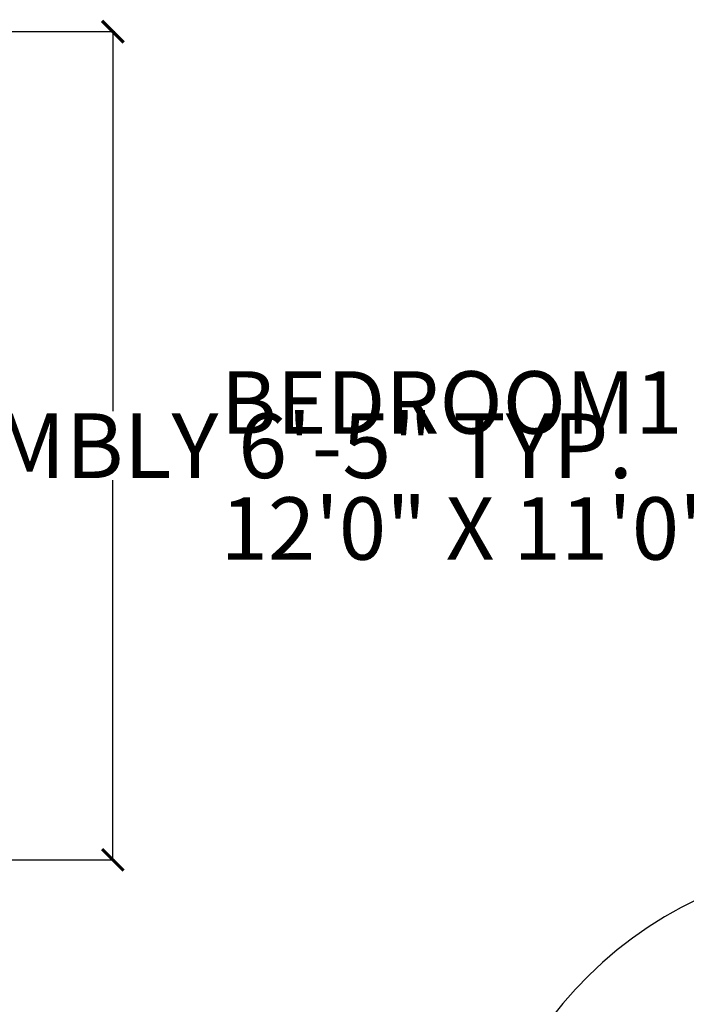
# Model space of a CAD drawing. Units: inches. Extents: x 528 to 2520, y -151 to 1354.
# Tile 6 of 41: x 658 to 720, y 1137 to 1229. Entities that reach past the tile are written whole.
import ezdxf

# ---------------------------------------------------------------- set-up
doc = ezdxf.new("R2010")
doc.units = ezdxf.units.IN
doc.header["$MEASUREMENT"] = 0
for name, color, linetype, lineweight in [('A-ANNO-DIMS', 2, 'Continuous', 18), ('A-AREA-IDEN', 7, 'Continuous', 18), ('A-Door', 150, 'Continuous', 25)]:
    doc.layers.add(name, color=color, linetype=linetype, lineweight=lineweight)
doc.layers.add('NT', color=1, linetype='Continuous')
doc.styles.get("Standard").update_dxf_attribs({"font": 'arial.ttf'})
doc.dimstyles.get("Standard").update_dxf_attribs({"dimtxt": 6, "dimasz": 2, "dimexe": 0.18, "dimexo": 0.0625, "dimgap": 0.09, "dimtad": 0, "dimtih": 1, "dimtoh": 1, "dimdec": 1, "dimzin": 0, "dimdsep": 46, "dimlunit": 3, "dimtxsty": 'Standard', "dimblk": 'ARCHTICK', "dimcen": 0.09, "dimadec": 0, "dimazin": 0, "dimtfac": 1, "dimtdec": 1, "dimtofl": 0, "dimtmove": 0, "dimatfit": 3, "dimfxl": 1, "dimtolj": 1, "dimtzin": 0, "dimarcsym": 0})

# ---------------------------------------------------------------- blocks, each defined once
blk = doc.blocks.new('A$C7DB75F4D')
at = {"layer": 'A-Door'}
for points in [[(625, 740), (625, 660), (665, 660), (665, 740)], [(625, 180), (625, 660), (665, 660), (665, 180)], [(625, 100), (625, 180), (665, 180), (665, 100)], [(35, 100), (35, 60), (50, 60), (50, 50), (50, 0), (0, 0), (0, 100)], [(665, 100), (700, 100), (700, 0), (650, 0), (650, 50), (650, 60), (665, 60)]]:
    blk.add_lwpolyline(points, close=True, dxfattribs=at)
at = {"layer": 'NT'}
blk.add_arc((650, 125), 615.5, 92.3278, 182.3278, dxfattribs=at)
blk = doc.blocks.new('_ArchTick')
at = {"color": 0, "linetype": 'ByBlock', "const_width": 0.15}
blk.add_lwpolyline([(-0.5, -0.5), (0.5, 0.5)], dxfattribs=at)
blk = doc.blocks.new('*D40')
at = {"layer": 'A-ANNO-DIMS', "color": 0, "lineweight": -2, "transparency": 16777216}
for p, q in [((744.634, 1150.503), (737.857, 1150.503)), ((738.037, 1150.503), (738.037, 1131.499)), ((738.037, 1106.103), (738.037, 1125.106)), ((744.634, 1106.103), (737.857, 1106.103))]:
    blk.add_line(p, q, dxfattribs=at)
at = {"layer": 'Defpoints', "color": 0, "transparency": 16777216}
for p in [(738.037, 1150.503), (744.697, 1150.503), (744.697, 1106.103)]:
    blk.add_point(p, dxfattribs=at)
at = {"layer": 'A-ANNO-DIMS', "color": 0, "lineweight": -2, "transparency": 16777216, "xscale": 2, "yscale": 2, "zscale": 2}
for p, rotation in [((738.037, 1150.503), 90), ((738.037, 1106.103), 270)]:
    blk.add_blockref('_ArchTick', p, dxfattribs=dict(at, rotation=rotation))
at = {"layer": 'A-ANNO-DIMS', "color": 0, "transparency": 16777216, "insert": (738.037, 1128.303), "char_height": 6, "attachment_point": 5}
blk.add_mtext('\\A1;DOOR SWING 3\'-8 1/2" TYP.', dxfattribs=at)
blk = doc.blocks.new('*D46')
at = {"layer": 'A-ANNO-DIMS', "color": 0, "lineweight": -2, "transparency": 16777216}
for p, q in [((655.184, 1227.431), (666.821, 1227.431)), ((666.641, 1227.431), (666.641, 1192.223)), ((666.641, 1150.631), (666.641, 1185.839)), ((655.184, 1150.631), (666.821, 1150.631))]:
    blk.add_line(p, q, dxfattribs=at)
at = {"layer": 'Defpoints', "color": 0, "transparency": 16777216}
for p in [(655.121, 1227.431), (666.641, 1227.431), (655.121, 1150.631)]:
    blk.add_point(p, dxfattribs=at)
at = {"layer": 'A-ANNO-DIMS', "color": 0, "lineweight": -2, "transparency": 16777216, "xscale": 2, "yscale": 2, "zscale": 2}
for p, rotation in [((666.641, 1227.431), 90), ((666.641, 1150.631), 270)]:
    blk.add_blockref('_ArchTick', p, dxfattribs=dict(at, rotation=rotation))
at = {"layer": 'A-ANNO-DIMS', "color": 0, "transparency": 16777216, "insert": (666.641, 1189.031), "char_height": 6, "attachment_point": 5}
blk.add_mtext('\\A1;BED ASSEMBLY 6\'-5" TYP.', dxfattribs=at)

msp = doc.modelspace()

# ---------------------------------------------------------------- block references
at = {"layer": 'A-Door', "xscale": 0.0600000000000059, "yscale": 0.0600000000000059, "zscale": 0.0600000000000059}
msp.add_blockref('A$C7DB75F4D', (697.697, 1106.103), dxfattribs=at)

# ---------------------------------------------------------------- texts
at = {"layer": 'A-AREA-IDEN'}
for s, height, p in [('BEDROOM1 ', 5.7926, (676.636, 1190.146)), ('12\'0" X 11\'0"', 5.79255, (676.636, 1178.46))]:
    msp.add_text(s, height=height, dxfattribs=at).set_placement(p)

# ---------------------------------------------------------------- dimensions: what is measured, and where the dimension line sits
at = {"layer": 'A-ANNO-DIMS'}
for base, p1, p2, text, picture, middle in [((666.641, 1227.431), (655.121, 1150.631), (655.121, 1227.431), 'BED ASSEMBLY <> TYP.', '*D46', (666.641, 1189.031)), ((738.037, 1150.503), (744.697, 1106.103), (744.697, 1150.503), 'DOOR SWING <> TYP.', '*D40', (738.037, 1128.303))]:
    dim = msp.add_linear_dim(base=base, p1=p1, p2=p2, angle=90, text=text, dimstyle='Standard', override={"dimdec": 1, "dimlfac": 1, "dimrnd": 0, "dimzin": 1, "dimdsep": 46, "dimlunit": 4, "dimfrac": 2}, dxfattribs=at)
    dim.commit()
    dim.dimension.update_dxf_attribs({"geometry": picture, "text_midpoint": middle})

doc.saveas('drawing.dxf')
